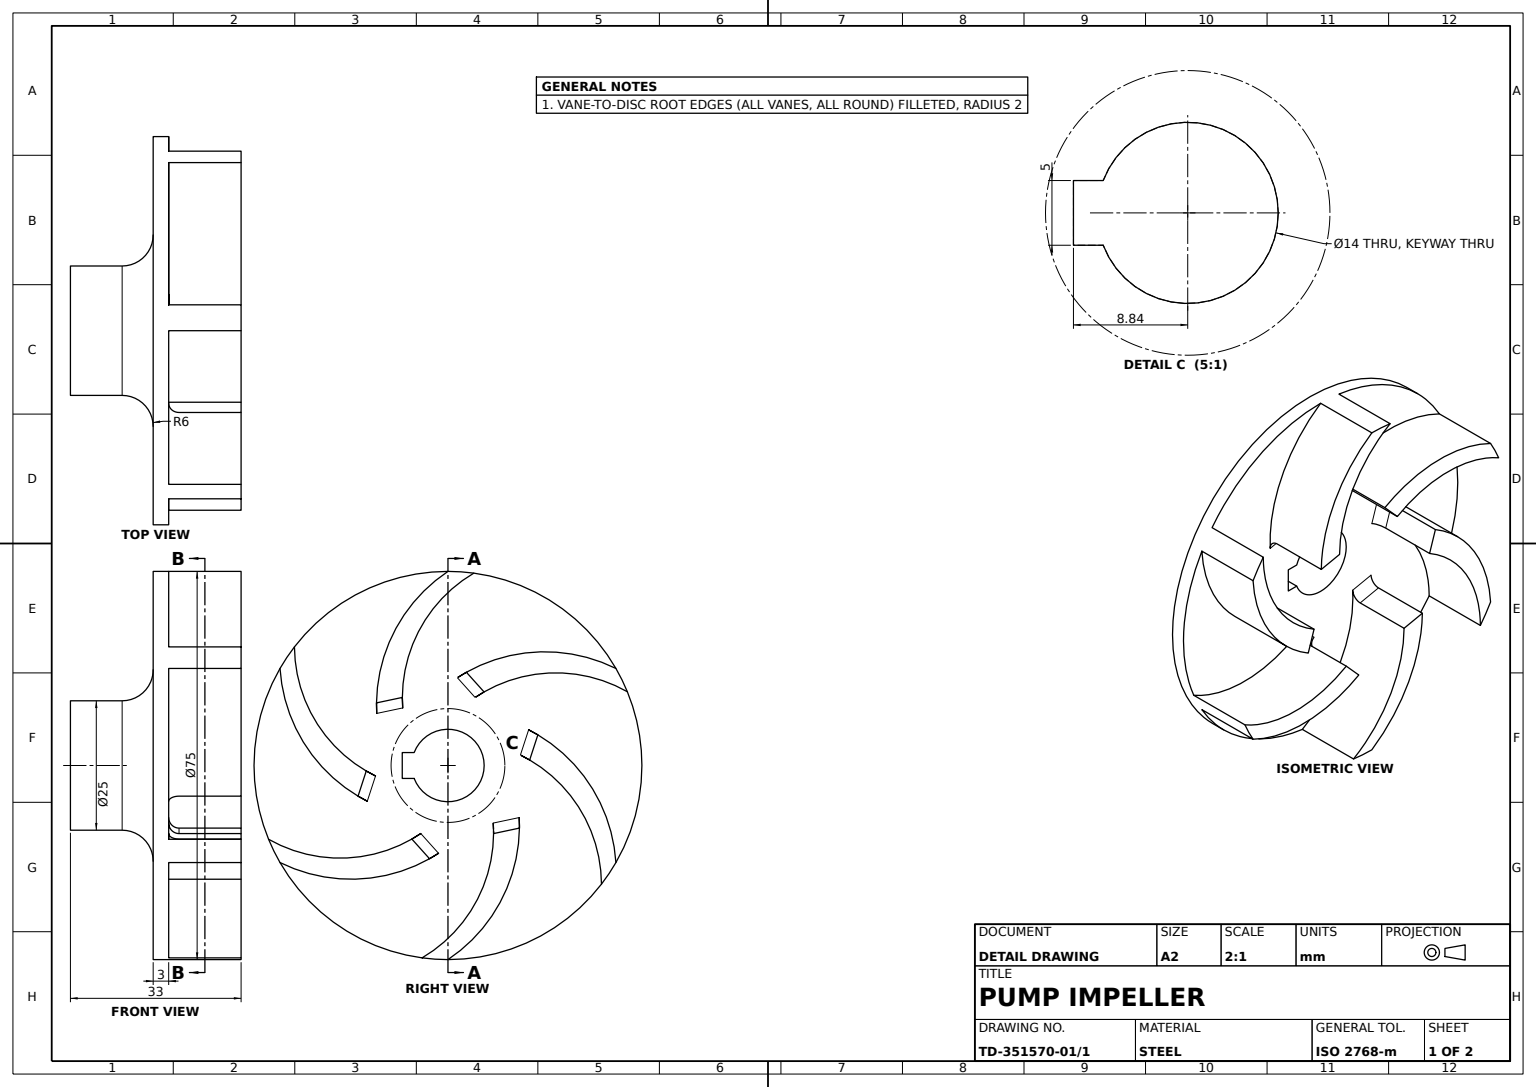
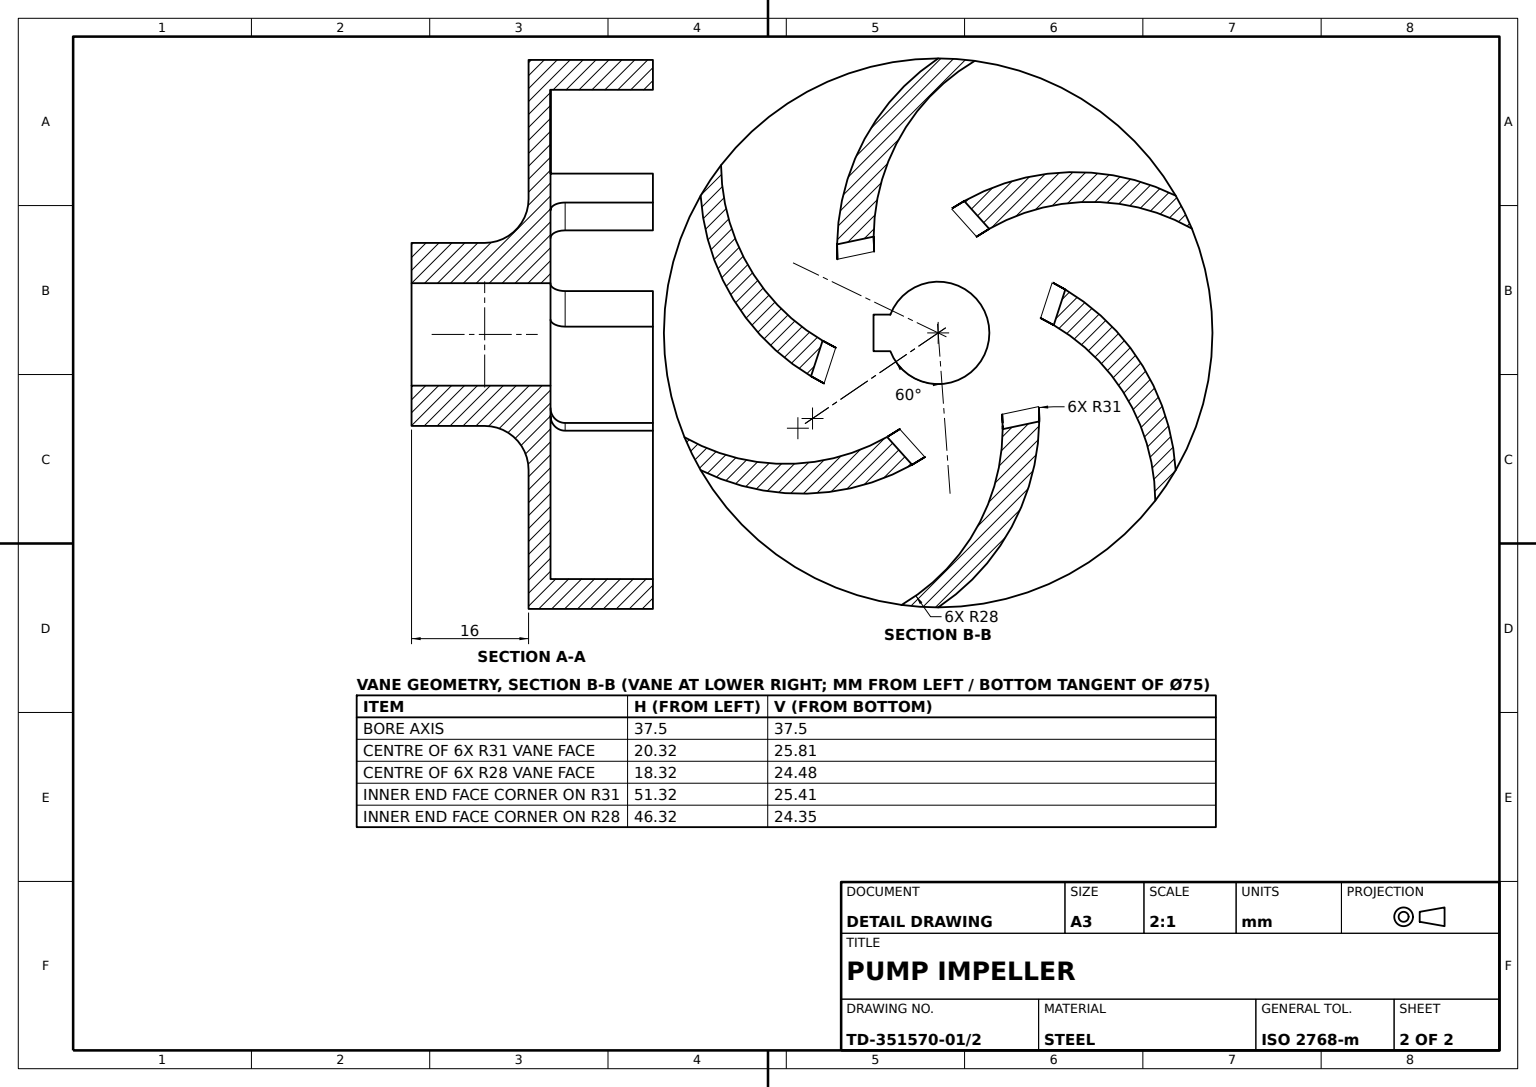
from build123d import *
from build123d.topology import SkipClean

# Parameters (mm, degrees)
BASE_DISC_SKETCH_75_R = 37.5
BASE_DISC_75X3_DEPTH  = 3
HUB_AND_BORE_SKETCH_R = 12.5
HUB_BOSS_DEPTH        = 16
SHAFT_BORE_DEPTH      = 23
HUB_FILLET_R6_R       = 6
VANES_6X_DEPTH        = 14
VANE_FILLETS_R2_R     = 2


with BuildPart() as part:
    # Base Disc Sketch _75 → Base Disc _75x3 (new body)
    with BuildSketch(Plane(origin=(0, 0, 0), x_dir=(1, 0, 0), z_dir=(0, 1, 0))):
        with Locations(Location((0, 0, 0), (0, 0, 270))):
            Circle(BASE_DISC_SKETCH_75_R)
    extrude(amount=BASE_DISC_75X3_DEPTH)

    # Hub and Bore Sketch → Hub Boss (add)
    with BuildSketch(Plane.XZ):
        with Locations(Location((0, 0, 0), (0, 0, 270))):
            Circle(HUB_AND_BORE_SKETCH_R)
    extrude(amount=HUB_BOSS_DEPTH)

    # Sketch2_3 → Shaft Bore (cut, symmetric)
    with BuildSketch(Plane.XZ):
        with BuildLine():
            Line((-2.5, 8.838348415), (2.5, 8.838348415))
            Line((2.5, 8.838348415), (2.5, 6.538348415))
            ThreePointArc((2.5, 6.538348415), (0, -7), (-2.5, 6.538348415))
            Line((-2.5, 6.538348415), (-2.5, 8.838348415))
        make_face()
    extrude(amount=SHAFT_BORE_DEPTH, both=True, mode=Mode.SUBTRACT)

    # Hub Fillet R6
    hub_fillet_r6_edges = [part.edges().sort_by_distance(p)[0] for p in [
        (0, 0, 12.5),
    ]]
    fillet(hub_fillet_r6_edges, radius=HUB_FILLET_R6_R)

    # Vane Profiles Sketch 6x → Vanes 6x (add)
    with SkipClean():  # the faces are left unmerged after this step: merging them gives an invalid solid
        with BuildSketch(Plane(origin=(0, 3, 0), x_dir=(1, 0, 0), z_dir=(0, 1, 0))):
            with BuildLine():
                Line((13.151074283, 8.81994991), (12.093810893, 13.81994991))
                ThreePointArc((12.093810893, 13.81994991), (26.507335187, 10.054378643), (37.5, 0))
                ThreePointArc((37.5, 0), (37.416199333, -2.505599224), (37.165171868, -5))
                ThreePointArc((37.165171868, -5), (26.987316196, 5.088454065), (13.151074283, 8.81994991))
            make_face()
            with BuildLine():
                Line((14.213837824, -6.979189461), (18.015333148, -3.563572506))
                ThreePointArc((18.015333148, -3.563572506), (21.961014917, -17.928836338), (18.75, -32.475952642))
                ThreePointArc((18.75, -32.475952642), (16.538187087, -33.656178747), (14.252458915, -34.685982974))
                ThreePointArc((14.252458915, -34.685982974), (17.900388584, -20.827474373), (14.213837824, -6.979189461))
            make_face()
            with BuildLine():
                Line((1.062763541, -15.799139371), (5.921522255, -17.383522417))
                ThreePointArc((5.921522255, -17.383522417), (-4.54632027, -27.98321498), (-18.75, -32.475952642))
                ThreePointArc((-18.75, -32.475952642), (-20.878012246, -31.150579524), (-22.912712953, -29.685982974))
                ThreePointArc((-22.912712953, -29.685982974), (-9.086927612, -25.915928438), (1.062763541, -15.799139371))
            make_face()
            with BuildLine():
                Line((-13.151074283, -8.81994991), (-12.093810893, -13.81994991))
                ThreePointArc((-12.093810893, -13.81994991), (-26.507335187, -10.054378643), (-37.5, 0))
                ThreePointArc((-37.5, 0), (-37.416199333, 2.505599224), (-37.165171868, 5))
                ThreePointArc((-37.165171868, 5), (-26.987316196, -5.088454065), (-13.151074283, -8.81994991))
            make_face()
            with BuildLine():
                Line((-14.213837824, 6.979189461), (-18.015333148, 3.563572506))
                ThreePointArc((-18.015333148, 3.563572506), (-21.961014917, 17.928836338), (-18.75, 32.475952642))
                ThreePointArc((-18.75, 32.475952642), (-16.538187087, 33.656178747), (-14.252458915, 34.685982974))
                ThreePointArc((-14.252458915, 34.685982974), (-17.900388584, 20.827474373), (-14.213837824, 6.979189461))
            make_face()
            with BuildLine():
                Line((-1.062763541, 15.799139371), (-5.921522255, 17.383522417))
                ThreePointArc((-5.921522255, 17.383522417), (4.54632027, 27.98321498), (18.75, 32.475952642))
                ThreePointArc((18.75, 32.475952642), (20.878012246, 31.150579524), (22.912712953, 29.685982974))
                ThreePointArc((22.912712953, 29.685982974), (9.086927612, 25.915928438), (-1.062763541, 15.799139371))
            make_face()
        extrude(amount=VANES_6X_DEPTH)

    # Vane Fillets R2
    vane_fillets_r2_edges = [part.edges().sort_by_distance(p)[0] for p in [
        (12.622442588, 3, -11.31994991),
        (16.114585486, 3, 5.271380984),
        (3.492142898, 3, 16.591330894),
        (-12.622442588, 3, 11.31994991),
        (-16.114585486, 3, -5.271380984),
        (-3.492142898, 3, -16.591330894),
    ]]
    fillet(vane_fillets_r2_edges, radius=VANE_FILLETS_R2_R)


solid = part.part
